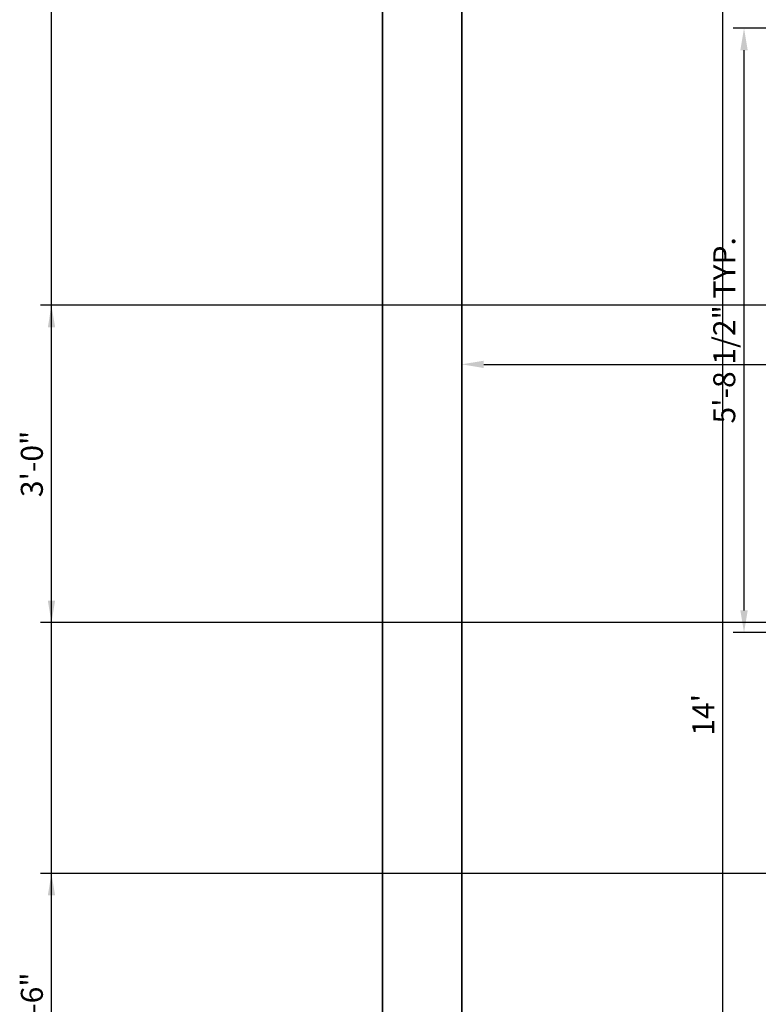
# Model space of a CAD drawing. Units: inches. Extents: x 2025 to 2528, y 1525 to 2336.
# Tile 9 of 18: x 2025 to 2109, y 2167 to 2278. Entities that reach past the tile are written whole.
import ezdxf

# ---------------------------------------------------------------- set-up
doc = ezdxf.new("R2010")
doc.units = ezdxf.units.IN
doc.layers.add('A-ANNO-DIMS', color=2, linetype='Continuous', lineweight=18)
doc.layers.add('A-WALL', color=7, linetype='Continuous', lineweight=35)
doc.styles.get("Standard").update_dxf_attribs({"font": 'arial.ttf'})
doc.dimstyles.new('Copy of ISO-25', dxfattribs={"dimtxt": 2.5, "dimasz": 2.5, "dimexe": 1.25, "dimexo": 0.625, "dimtad": 1, "dimdec": 1, "dimlunit": 4, "dimtxsty": 'Standard', "dimcen": 2.5, "dimadec": 0, "dimazin": 0, "dimtfac": 1, "dimtdec": 1, "dimtmove": 0, "dimatfit": 3, "dimfxl": 1, "dimarcsym": 0})

# ---------------------------------------------------------------- blocks, each defined once
blk = doc.blocks.new('*D6')
at = {"layer": 'A-ANNO-DIMS', "color": 0, "lineweight": -2, "transparency": 16777216}
for p, q in [((2075.01, 2282.79), (2075.01, 2237.93)), ((2255.01, 2282.79), (2255.01, 2237.93)), ((2077.51, 2239.18), (2252.51, 2239.18))]:
    blk.add_line(p, q, dxfattribs=at)
at = {"layer": 'A-ANNO-DIMS', "color": 0, "transparency": 16777216}
for points in [[(2077.51, 2239.59), (2077.51, 2238.76), (2075.01, 2239.18)], [(2252.51, 2239.59), (2252.51, 2238.76), (2255.01, 2239.18)]]:
    blk.add_solid(points, dxfattribs=at)
at = {"layer": 'Defpoints', "color": 0, "transparency": 16777216}
for p in [(2075.01, 2283.41), (2255.01, 2283.41), (2255.01, 2239.18)]:
    blk.add_point(p, dxfattribs=at)
at = {"layer": 'A-ANNO-DIMS', "color": 0, "transparency": 16777216, "insert": (2165.01, 2241.08), "char_height": 2.5, "attachment_point": 5}
blk.add_mtext("15'", dxfattribs=at)
blk = doc.blocks.new('*D7')
at = {"layer": 'A-ANNO-DIMS', "color": 0, "lineweight": -2, "transparency": 16777216}
for p, q in [((2075.64, 2283.41), (2105.88, 2283.41)), ((2104.63, 2117.91), (2104.63, 2280.91)), ((2075.64, 2115.41), (2105.88, 2115.41))]:
    blk.add_line(p, q, dxfattribs=at)
at = {"layer": 'A-ANNO-DIMS', "color": 0, "transparency": 16777216}
for points in [[(2104.22, 2280.91), (2105.05, 2280.91), (2104.63, 2283.41)], [(2104.22, 2117.91), (2105.05, 2117.91), (2104.63, 2115.41)]]:
    blk.add_solid(points, dxfattribs=at)
at = {"layer": 'Defpoints', "color": 0, "transparency": 16777216}
for p in [(2075.01, 2283.41), (2104.63, 2283.41), (2075.01, 2115.41)]:
    blk.add_point(p, dxfattribs=at)
at = {"layer": 'A-ANNO-DIMS', "color": 0, "transparency": 16777216, "insert": (2102.75, 2199.41), "char_height": 2.5, "attachment_point": 5, "rotation": 90}
blk.add_mtext("14'", dxfattribs=at)
blk = doc.blocks.new('*D57')
at = {"layer": 'A-ANNO-DIMS', "color": 0, "lineweight": -2, "transparency": 16777216}
for p, q in [((2119.58, 2277.32), (2105.8, 2277.32)), ((2107.05, 2211.26), (2107.05, 2274.82)), ((2119.58, 2208.76), (2105.8, 2208.76))]:
    blk.add_line(p, q, dxfattribs=at)
at = {"layer": 'A-ANNO-DIMS', "color": 0, "transparency": 16777216}
for points in [[(2106.63, 2274.82), (2107.47, 2274.82), (2107.05, 2277.32)], [(2106.63, 2211.26), (2107.47, 2211.26), (2107.05, 2208.76)]]:
    blk.add_solid(points, dxfattribs=at)
at = {"layer": 'Defpoints', "color": 0, "transparency": 16777216}
for p in [(2107.05, 2277.32), (2120.21, 2277.32), (2120.21, 2208.76)]:
    blk.add_point(p, dxfattribs=at)
at = {"layer": 'A-ANNO-DIMS', "color": 0, "transparency": 16777216, "insert": (2105.13, 2243.04), "char_height": 2.5, "attachment_point": 5, "rotation": 90}
blk.add_mtext('5\'-8 1/2" TYP.', dxfattribs=at)
blk = doc.blocks.new('*D77')
at = {"layer": 'A-ANNO-DIMS', "color": 0, "lineweight": -2, "transparency": 16777216}
for p, q in [((2254.39, 2181.41), (2027.21, 2181.41)), ((2028.46, 2153.91), (2028.46, 2178.91)), ((2254.39, 2151.41), (2027.21, 2151.41))]:
    blk.add_line(p, q, dxfattribs=at)
at = {"layer": 'A-ANNO-DIMS', "color": 0, "transparency": 16777216}
for points in [[(2028.05, 2178.91), (2028.88, 2178.91), (2028.46, 2181.41)], [(2028.05, 2153.91), (2028.88, 2153.91), (2028.46, 2151.41)]]:
    blk.add_solid(points, dxfattribs=at)
at = {"layer": 'Defpoints', "color": 0, "transparency": 16777216}
for p in [(2028.46, 2181.41), (2255.01, 2181.41), (2255.01, 2151.41)]:
    blk.add_point(p, dxfattribs=at)
at = {"layer": 'A-ANNO-DIMS', "color": 0, "transparency": 16777216, "insert": (2026.56, 2166.41), "char_height": 2.5, "attachment_point": 5, "rotation": 90}
blk.add_mtext('2\'-6"', dxfattribs=at)
blk = doc.blocks.new('*D78')
at = {"layer": 'A-ANNO-DIMS', "color": 0, "lineweight": -2, "transparency": 16777216}
for p, q in [((2254.39, 2245.88), (2027.21, 2245.88)), ((2028.46, 2212.38), (2028.46, 2243.38)), ((2254.39, 2209.88), (2027.21, 2209.88))]:
    blk.add_line(p, q, dxfattribs=at)
at = {"layer": 'A-ANNO-DIMS', "color": 0, "transparency": 16777216}
for points in [[(2028.05, 2243.38), (2028.88, 2243.38), (2028.46, 2245.88)], [(2028.05, 2212.38), (2028.88, 2212.38), (2028.46, 2209.88)]]:
    blk.add_solid(points, dxfattribs=at)
at = {"layer": 'Defpoints', "color": 0, "transparency": 16777216}
for p in [(2028.46, 2245.88), (2255.01, 2245.88), (2255.01, 2209.88)]:
    blk.add_point(p, dxfattribs=at)
at = {"layer": 'A-ANNO-DIMS', "color": 0, "transparency": 16777216, "insert": (2026.56, 2227.88), "char_height": 2.5, "attachment_point": 5, "rotation": 90}
blk.add_mtext('3\'-0"', dxfattribs=at)
blk = doc.blocks.new('*D80')
at = {"layer": 'A-ANNO-DIMS', "color": 0, "lineweight": -2, "transparency": 16777216}
for p, q in [((2065.39, 2292.41), (2027.21, 2292.41)), ((2028.46, 1566.91), (2028.46, 2289.91)), ((2285.39, 1564.41), (2027.21, 1564.41))]:
    blk.add_line(p, q, dxfattribs=at)
at = {"layer": 'A-ANNO-DIMS', "color": 0, "transparency": 16777216}
for points in [[(2028.05, 2289.91), (2028.88, 2289.91), (2028.46, 2292.41)], [(2028.05, 1566.91), (2028.88, 1566.91), (2028.46, 1564.41)]]:
    blk.add_solid(points, dxfattribs=at)
at = {"layer": 'Defpoints', "color": 0, "transparency": 16777216}
for p in [(2028.46, 2292.41), (2066.01, 2292.41), (2286.01, 1564.41)]:
    blk.add_point(p, dxfattribs=at)
at = {"layer": 'A-ANNO-DIMS', "color": 0, "transparency": 16777216, "insert": (2026.56, 1928.41), "char_height": 2.5, "attachment_point": 5, "rotation": 90}
blk.add_mtext('60\'-8"', dxfattribs=at)

msp = doc.modelspace()

# ---------------------------------------------------------------- linework, layer by layer
at = {"layer": 'A-WALL'}
for p, q in [((2066.01, 2283.41), (2066.01, 2115.41)), ((2075.01, 2283.41), (2075.01, 2115.41)), ((2075.01, 2283.41), (2075.01, 2115.41))]:
    msp.add_line(p, q, dxfattribs=at)

# ---------------------------------------------------------------- dimensions: what is measured, and where the dimension line sits
at = {"layer": 'A-ANNO-DIMS'}
for base, p1, p2, override, picture, middle in [((2028.46, 2292.41), (2286.01, 1564.41), (2066.01, 2292.41), {"dimdec": 1, "dimlfac": 1, "dimrnd": 0, "dimzin": 1, "dimdsep": 46, "dimlunit": 4, "dimfrac": 2}, '*D80', (2026.56, 1928.41)), ((2104.63, 2283.41), (2075.01, 2115.41), (2075.01, 2283.41), {"dimclrd": 0, "dimclre": 0, "dimclrt": 0}, '*D7', (2102.75, 2199.41)), ((2028.46, 2245.88), (2255.01, 2209.88), (2255.01, 2245.88), {"dimdec": 1, "dimlfac": 1, "dimrnd": 0, "dimzin": 1, "dimdsep": 46, "dimlunit": 4, "dimfrac": 2}, '*D78', (2026.56, 2227.88)), ((2028.46, 2181.41), (2255.01, 2151.41), (2255.01, 2181.41), {"dimdec": 1, "dimlfac": 1, "dimrnd": 0, "dimzin": 1, "dimdsep": 46, "dimlunit": 4, "dimfrac": 2}, '*D77', (2026.56, 2166.41))]:
    dim = msp.add_linear_dim(base=base, p1=p1, p2=p2, angle=90, dimstyle='Copy of ISO-25', override=override, dxfattribs=at)
    dim.commit()
    dim.dimension.update_dxf_attribs({"geometry": picture, "text_midpoint": middle})
dim = msp.add_linear_dim(base=(2255.01, 2239.18), p1=(2075.01, 2283.41), p2=(2255.01, 2283.41), dimstyle='Copy of ISO-25', override={"dimclrd": 0, "dimclre": 0, "dimclrt": 0}, dxfattribs=at)
dim.commit()
dim.dimension.update_dxf_attribs({"geometry": '*D6', "text_midpoint": (2165.01, 2241.08)})
dim = msp.add_linear_dim(base=(2107.05, 2277.32), p1=(2120.21, 2208.76), p2=(2120.21, 2277.32), angle=90, text='<> TYP.', dimstyle='Copy of ISO-25', override={"dimdec": 1, "dimlfac": 1, "dimrnd": 0, "dimzin": 1, "dimdsep": 46, "dimlunit": 4, "dimfrac": 2}, dxfattribs=at)
dim.commit()
dim.dimension.update_dxf_attribs({"geometry": '*D57', "text_midpoint": (2105.13, 2243.04)})

doc.saveas('drawing.dxf')
